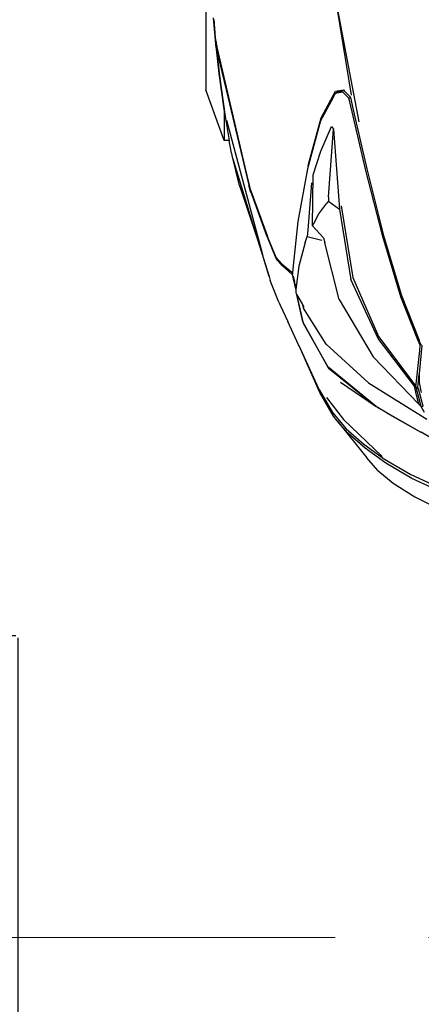
# Model space of a CAD drawing. Units: inches. Extents: x 0 to 4258, y 0 to 3769.
# Tile 5 of 30: x 3726 to 3739, y 2971 to 3003. Entities that reach past the tile are written whole.
import ezdxf

# ---------------------------------------------------------------- set-up
doc = ezdxf.new("R2010")
doc.units = ezdxf.units.IN
doc.header["$MEASUREMENT"] = 0
doc.linetypes.add('ACAD_ISO02W100', pattern=[15, 12, -3])
doc.layers.get('0').update_dxf_attribs({"color": 16})
for name, color, linetype, lineweight in [('A-ANNO-DIMS', 250, 'Continuous', 18), ('A-FLOR-OVHD', 150, 'ACAD_ISO02W100', 13), ('C-PKNG-VEHI', 8, 'Continuous', 18)]:
    doc.layers.add(name, color=color, linetype=linetype, lineweight=lineweight)
doc.layers.add('Edges', color=250, linetype='Continuous')
doc.styles.get("Standard").update_dxf_attribs({"font": 'arial.ttf'})
doc.dimstyles.get("Standard").update_dxf_attribs({"dimtxt": 7, "dimasz": 0.18, "dimexe": 0.18, "dimexo": 0.0625, "dimgap": 0.09, "dimtad": 0, "dimtih": 1, "dimtoh": 1, "dimzin": 0, "dimdsep": 46, "dimlunit": 3, "dimtxsty": 'Standard', "dimcen": 0.09, "dimadec": 0, "dimazin": 0, "dimtfac": 1, "dimtofl": 0, "dimtmove": 0, "dimatfit": 3, "dimfxl": 1, "dimtolj": 1, "dimtzin": 0, "dimarcsym": 0})

# ---------------------------------------------------------------- blocks, each defined once
blk = doc.blocks.new('Nissan Qashqai pl')
at = {"layer": 'Edges'}
for p, q in [((11.47322, 11.2592), (11.46579, 11.24614)), ((11.50736, 11.23616), (11.51652, 11.25601)), ((11.52058, 11.25724), (11.51126, 11.23721)), ((11.52949, 11.24004), (11.53843, 11.2583)), ((11.33108, 11.22699), (11.37506, 11.24429)), ((11.37475, 11.24309), (11.33228, 11.22637)), ((11.38, 11.24532), (11.37475, 11.24309)), ((11.37506, 11.24429), (11.37524, 11.24436)), ((11.37506, 11.24429), (11.37621, 11.24429)), ((11.37922, 11.24593), (11.37524, 11.24436)), ((11.3763, 11.24436), (11.37524, 11.24436)), ((11.37922, 11.24593), (11.38041, 11.24692)), ((11.37933, 11.24631), (11.37922, 11.24593)), ((11.38533, 11.24487), (11.38, 11.24532)), ((11.38041, 11.24692), (11.40818, 11.24436)), ((11.42115, 11.24117), (11.38533, 11.24487)), ((11.3915, 11.19885), (11.4381, 11.24397)), ((11.41644, 11.24436), (11.40818, 11.24436)), ((11.40898, 11.24429), (11.40818, 11.24436)), ((11.40898, 11.24429), (11.4163, 11.24429)), ((11.4152, 11.24371), (11.40898, 11.24429)), ((11.4163, 11.24429), (11.4152, 11.24371)), ((11.42154, 11.24313), (11.4152, 11.24371)), ((11.41644, 11.24436), (11.4163, 11.24429)), ((11.41686, 11.24458), (11.41644, 11.24436)), ((11.4252, 11.2462), (11.41686, 11.24458)), ((11.41698, 11.19425), (11.45295, 11.25195)), ((11.42115, 11.24117), (11.42154, 11.24313)), ((11.42296, 11.24352), (11.42154, 11.24313)), ((11.43154, 11.24397), (11.42287, 11.24164)), ((11.42296, 11.24352), (11.42287, 11.24164)), ((11.43996, 11.24823), (11.42296, 11.24352)), ((11.42659, 11.2465), (11.4252, 11.2462)), ((11.4381, 11.24397), (11.42915, 11.24177)), ((11.44027, 11.24637), (11.43154, 11.24397)), ((11.4381, 11.24397), (11.44027, 11.24637)), ((11.44027, 11.24637), (11.43996, 11.24823)), ((11.44624, 11.24948), (11.44027, 11.24637)), ((11.44114, 11.20281), (11.46562, 11.24583)), ((11.44697, 11.21272), (11.46562, 11.24583)), ((11.46562, 11.24583), (11.46579, 11.24614)), ((11.3715, 11.20434), (11.41772, 11.23895)), ((11.42033, 11.23975), (11.37334, 11.20375)), ((11.41772, 11.23895), (11.41931, 11.23998)), ((11.41915, 11.23969), (11.4194, 11.23996)), ((11.41931, 11.23998), (11.4196, 11.24017)), ((11.4194, 11.23996), (11.41931, 11.23998)), ((11.4194, 11.23996), (11.4196, 11.24017)), ((11.41958, 11.23992), (11.4194, 11.23996)), ((11.4196, 11.24017), (11.42014, 11.24052)), ((11.41984, 11.24006), (11.42014, 11.24052)), ((11.42014, 11.24052), (11.42115, 11.24117)), ((11.42915, 11.24177), (11.42033, 11.23975)), ((11.42287, 11.24164), (11.42033, 11.23975)), ((11.42178, 11.24134), (11.42115, 11.24117)), ((11.42287, 11.24164), (11.42178, 11.24134)), ((11.42216, 11.24127), (11.42178, 11.24134)), ((11.49236, 11.21027), (11.50736, 11.23616)), ((11.51126, 11.23721), (11.49628, 11.21137)), ((11.51576, 11.21859), (11.52949, 11.24004)), ((11.27199, 11.20923), (11.33108, 11.22699)), ((11.33228, 11.22637), (11.27276, 11.20843)), ((11.50327, 11.20341), (11.51576, 11.21859)), ((11.20627, 11.19262), (11.27199, 11.20923)), ((11.27276, 11.20843), (11.20665, 11.19145)), ((11.31316, 11.17892), (11.3715, 11.20434)), ((11.37334, 11.20375), (11.31527, 11.17691)), ((11.44697, 11.21272), (11.44114, 11.20281)), ((11.45306, 11.16974), (11.48975, 11.20767)), ((11.47745, 11.18983), (11.49236, 11.21027)), ((11.49628, 11.21137), (11.48154, 11.19102)), ((11.33497, 11.16556), (11.3915, 11.19885)), ((11.37896, 11.15265), (11.41698, 11.19425)), ((11.44046, 11.20182), (11.40144, 11.15414)), ((11.40216, 11.15476), (11.44046, 11.20182)), ((11.41633, 11.16662), (11.44046, 11.20182)), ((11.44081, 11.20225), (11.44046, 11.20182)), ((11.4411, 11.20277), (11.44081, 11.20225)), ((11.44114, 11.20281), (11.4411, 11.20277)), ((11.49363, 11.19502), (11.49082, 11.19282)), ((11.50327, 11.20341), (11.49363, 11.19502)), ((11.03575, 11.16129), (11.1598, 11.18473)), ((11.20665, 11.19145), (11.14012, 11.17593)), ((11.14803, 11.17913), (11.20627, 11.19262)), ((11.45433, 11.16358), (11.49082, 11.19282)), ((11.46237, 11.17248), (11.47745, 11.18983)), ((11.48154, 11.19102), (11.46617, 11.17358)), ((11.04919, 11.16347), (11.13359, 11.17719)), ((11.12929, 11.17052), (11.13526, 11.17642)), ((11.13658, 11.17502), (11.1347, 11.17313)), ((11.13526, 11.17642), (11.13585, 11.17654)), ((11.13585, 11.17654), (11.14803, 11.17913)), ((11.13585, 11.17654), (11.13658, 11.17502)), ((11.14012, 11.17593), (11.13658, 11.17502)), ((11.24278, 11.16729), (11.31316, 11.17892)), ((11.24587, 11.16563), (11.31527, 11.17691)), ((11.12846, 11.16971), (11.12929, 11.17052)), ((11.12977, 11.16183), (11.12846, 11.16971)), ((11.12929, 11.17052), (11.13057, 11.16299)), ((11.1347, 11.17313), (11.13062, 11.16899)), ((11.13062, 11.16899), (11.13192, 11.16144)), ((11.16717, 11.15976), (11.24587, 11.16563)), ((11.23823, 11.15494), (11.24587, 11.16563)), ((11.33497, 11.16556), (11.27913, 11.15147)), ((11.43143, 11.15309), (11.45306, 11.16974)), ((11.44642, 11.15882), (11.46237, 11.17248)), ((11.46617, 11.17358), (11.45433, 11.16358)), ((11.15597, 11.14759), (11.12977, 11.16183)), ((11.13192, 11.16144), (11.13057, 11.16299)), ((11.13192, 11.16144), (11.13652, 11.15905)), ((11.13652, 11.15905), (11.15893, 11.14704)), ((11.16444, 11.15792), (11.16717, 11.15976)), ((11.18896, 11.14734), (11.16444, 11.15792)), ((11.23369, 11.15498), (11.16717, 11.15976)), ((11.42433, 11.14593), (11.44642, 11.15882)), ((11.44983, 11.15977), (11.42671, 11.14629)), ((11.45433, 11.16358), (11.44983, 11.15977)), ((11.20291, 11.13489), (11.15597, 11.14759)), ((11.15893, 11.14704), (11.20616, 11.13437)), ((11.2121, 11.1399), (11.18896, 11.14734)), ((11.23369, 11.15498), (11.23823, 11.15494)), ((11.23823, 11.15494), (11.2401, 11.15337)), ((11.25046, 11.1455), (11.2401, 11.15337)), ((11.26005, 11.1405), (11.25046, 11.1455)), ((11.27429, 11.14993), (11.26224, 11.13901)), ((11.27289, 11.13379), (11.27664, 11.14845)), ((11.27429, 11.14993), (11.27913, 11.15147)), ((11.37896, 11.15265), (11.34336, 11.13032)), ((11.40144, 11.15414), (11.3571, 11.12956)), ((11.35832, 11.12998), (11.40144, 11.15414)), ((11.42671, 11.14629), (11.38067, 11.12595)), ((11.40216, 11.15476), (11.40144, 11.15414)), ((11.42283, 11.14525), (11.42433, 11.14593)), ((11.26224, 11.13901), (11.2121, 11.1399)), ((11.21991, 11.1382), (11.26663, 11.13449)), ((11.26224, 11.13901), (11.26005, 11.1405)), ((11.42283, 11.14525), (11.38067, 11.12595)), ((11.20291, 11.13489), (11.20295, 11.13488)), ((11.20295, 11.13488), (11.20616, 11.13437)), ((11.20616, 11.13437), (11.25827, 11.12461)), ((11.26663, 11.13449), (11.27289, 11.13379)), ((11.27871, 11.13184), (11.27289, 11.13379)), ((11.27871, 11.13184), (11.30218, 11.1256)), ((11.32955, 11.12347), (11.3571, 11.12956)), ((11.3571, 11.12956), (11.33021, 11.12384)), ((11.33021, 11.12384), (11.33938, 11.12898)), ((11.33938, 11.12898), (11.34202, 11.13045)), ((11.33938, 11.12898), (11.34336, 11.13032)), ((11.3571, 11.12956), (11.35832, 11.12998)), ((11.25827, 11.12461), (11.29558, 11.12077)), ((11.29558, 11.12077), (11.30849, 11.1195)), ((11.30003, 11.10916), (11.30813, 11.11883)), ((11.31027, 11.11923), (11.30178, 11.10961)), ((11.30218, 11.1256), (11.32517, 11.12286)), ((11.30805, 11.11884), (11.30863, 11.11948)), ((11.30813, 11.11883), (11.30863, 11.11948)), ((11.30849, 11.1195), (11.30863, 11.11948)), ((11.30863, 11.11948), (11.31033, 11.1193)), ((11.31033, 11.1193), (11.31027, 11.11923)), ((11.31033, 11.1193), (11.31061, 11.11927)), ((11.31061, 11.11927), (11.314, 11.12039)), ((11.31704, 11.12142), (11.31186, 11.12058)), ((11.31323, 11.11986), (11.32588, 11.12266)), ((11.32423, 11.12258), (11.314, 11.12039)), ((11.314, 11.12039), (11.31704, 11.12142)), ((11.32423, 11.12258), (11.31704, 11.12142)), ((11.31982, 11.1231), (11.32517, 11.12286)), ((11.32423, 11.12258), (11.32588, 11.12266)), ((11.32517, 11.12286), (11.32831, 11.12278)), ((11.32588, 11.12266), (11.32831, 11.12278)), ((11.32831, 11.12278), (11.32955, 11.12347)), ((11.32955, 11.12347), (11.33021, 11.12384)), ((11.37962, 11.12547), (11.35656, 11.11477)), ((11.38067, 11.12595), (11.37962, 11.12547)), ((11.29339, 11.10313), (11.30003, 11.10916)), ((11.30178, 11.10961), (11.29459, 11.10327)), ((11.33757, 11.10603), (11.34052, 11.10725)), ((11.34052, 11.10725), (11.35656, 11.11477)), ((11.29459, 11.10327), (11.27358, 11.0947)), ((11.27407, 11.09522), (11.29339, 11.10313)), ((11.31244, 11.09628), (11.31612, 11.09747)), ((11.33757, 11.10603), (11.31612, 11.09747)), ((11.15816, 11.05423), (11.29065, 11.08989)), ((11.2732, 11.09452), (11.22772, 11.07792)), ((11.23038, 11.07923), (11.27187, 11.09432)), ((11.27187, 11.09432), (11.27407, 11.09522)), ((11.27358, 11.0947), (11.2732, 11.09452)), ((11.27358, 11.0947), (11.27407, 11.09522)), ((11.27568, 11.08503), (11.31244, 11.09628)), ((11.31244, 11.09628), (11.29065, 11.08989)), ((11.30801, 11.09508), (11.30877, 11.09528)), ((11.19633, 11.06072), (11.27568, 11.08503)), ((11.22715, 11.07771), (11.2222, 11.07656)), ((11.22475, 11.06772), (11.27568, 11.08503)), ((11.22532, 11.07737), (11.23038, 11.07923)), ((11.22731, 11.07783), (11.22706, 11.07777)), ((11.22962, 11.07837), (11.22715, 11.07771)), ((11.22772, 11.07792), (11.22715, 11.07771)), ((11.22962, 11.07837), (11.22772, 11.07792)), ((11.08649, 11.04496), (11.21998, 11.07614)), ((11.22216, 11.0766), (11.08821, 11.045)), ((11.09177, 11.04531), (11.22216, 11.0766)), ((11.21998, 11.07614), (11.22216, 11.0766)), ((11.2222, 11.07656), (11.22216, 11.0766)), ((11.22238, 11.07665), (11.2222, 11.07656)), ((11.22238, 11.07665), (11.22532, 11.07737)), ((11.19065, 11.05923), (11.17828, 11.05716)), ((11.19089, 11.05929), (11.19065, 11.05923)), ((11.19089, 11.05929), (11.19297, 11.05964)), ((11.19297, 11.05964), (11.22148, 11.06662)), ((11.22148, 11.06662), (11.22475, 11.06772)), ((11.14751, 11.05208), (11.11234, 11.04716)), ((11.11474, 11.04762), (11.15472, 11.05317)), ((11.17828, 11.05208), (11.12828, 11.03408)), ((11.15248, 11.05278), (11.14751, 11.05208)), ((11.14751, 11.05208), (11.17828, 11.05208)), ((11.15472, 11.05317), (11.15248, 11.05278)), ((11.15472, 11.05317), (11.17828, 11.05716)), ((11.17828, 11.05716), (11.17828, 11.05208)), ((11.07977, 11.04339), (11.05762, 11.04159)), ((11.05899, 11.04188), (11.07681, 11.04337)), ((11.07681, 11.04337), (11.08106, 11.04371)), ((11.08696, 11.04422), (11.07977, 11.04339)), ((11.08106, 11.04371), (11.08273, 11.0441)), ((11.08114, 11.04436), (11.08208, 11.0442)), ((11.08273, 11.0441), (11.08562, 11.04476)), ((11.08273, 11.0441), (11.08365, 11.04395)), ((11.08821, 11.045), (11.08365, 11.04395)), ((11.08365, 11.04395), (11.08696, 11.04422)), ((11.08562, 11.04476), (11.08649, 11.04496)), ((11.08649, 11.04496), (11.08796, 11.04514)), ((11.08696, 11.04422), (11.08721, 11.04424)), ((11.08728, 11.04426), (11.08721, 11.04424)), ((11.08728, 11.04426), (11.08834, 11.04438)), ((11.08834, 11.04438), (11.11474, 11.04762)), ((11.11234, 11.04716), (11.08834, 11.04438)), ((10.95773, 11.03408), (11.12828, 11.03408))]:
    blk.add_line(p, q, dxfattribs=at)
blk = doc.blocks.new('car')
blk.add_blockref('Nissan Qashqai pl', (-9.74328, -11.91512))
blk = doc.blocks.new('*D66')
at = {"layer": 'A-ANNO-DIMS', "color": 0, "lineweight": -2, "transparency": 16777216}
for p, q in [((3725.517, 3125.846), (3703.936, 3125.846)), ((3704.116, 3125.666), (3704.116, 3058.01)), ((3704.116, 2982.935), (3704.116, 3050.591)), ((3725.517, 2982.755), (3703.936, 2982.755))]:
    blk.add_line(p, q, dxfattribs=at)
at = {"layer": 'A-ANNO-DIMS', "color": 0, "transparency": 16777216}
for points in [[(3704.086, 3125.666), (3704.146, 3125.666), (3704.116, 3125.846)], [(3704.086, 2982.935), (3704.146, 2982.935), (3704.116, 2982.755)]]:
    blk.add_solid(points, dxfattribs=at)
at = {"layer": 'Defpoints', "color": 0, "transparency": 16777216}
for p in [(3725.58, 3125.846), (3704.116, 2982.755), (3725.58, 2982.755)]:
    blk.add_point(p, dxfattribs=at)
at = {"layer": 'A-ANNO-DIMS', "color": 0, "transparency": 16777216, "insert": (3704.116, 3054.301), "char_height": 7, "attachment_point": 5}
blk.add_mtext('\\A1;CAR 11\'-11"', dxfattribs=at)
blk = doc.blocks.new('*D67')
at = {"layer": 'A-ANNO-DIMS', "color": 0, "lineweight": -2, "transparency": 16777216}
for p, q in [((3725.58, 2982.693), (3725.58, 2961.112)), ((3795.713, 2982.693), (3795.713, 2961.112)), ((3725.76, 2961.292), (3748.533, 2961.292)), ((3795.533, 2961.292), (3772.76, 2961.292))]:
    blk.add_line(p, q, dxfattribs=at)
at = {"layer": 'A-ANNO-DIMS', "color": 0, "transparency": 16777216}
for points in [[(3725.76, 2961.322), (3725.76, 2961.262), (3725.58, 2961.292)], [(3795.533, 2961.322), (3795.533, 2961.262), (3795.713, 2961.292)]]:
    blk.add_solid(points, dxfattribs=at)
at = {"layer": 'Defpoints', "color": 0, "transparency": 16777216}
for p in [(3725.58, 2982.755), (3795.713, 2982.755), (3795.713, 2961.292)]:
    blk.add_point(p, dxfattribs=at)
at = {"layer": 'A-ANNO-DIMS', "color": 0, "transparency": 16777216, "insert": (3760.646, 2961.292), "char_height": 7, "attachment_point": 5}
blk.add_mtext('\\A1;5\'-10"', dxfattribs=at)

msp = doc.modelspace()

# ---------------------------------------------------------------- linework, layer by layer
at = {"layer": 'A-FLOR-OVHD'}
msp.add_line((3678.804, 2973.052), (3832.744, 2973.052), dxfattribs=at)

# ---------------------------------------------------------------- block references
at = {"layer": 'C-PKNG-VEHI', "xscale": 32.66500240257601, "yscale": 32.66500240257601, "zscale": 32.66500240257601, "rotation": 270}
msp.add_blockref('car', (3760.419, 3045.57), dxfattribs=at)

# ---------------------------------------------------------------- dimensions: what is measured, and where the dimension line sits
at = {"layer": 'A-ANNO-DIMS'}
dim = msp.add_linear_dim(base=(3704.116, 2982.755), p1=(3725.58, 3125.846), p2=(3725.58, 2982.755), angle=270, text='CAR <>', dimstyle='Standard', override={"dimdec": 1, "dimlfac": 1, "dimrnd": 0, "dimzin": 1, "dimdsep": 46, "dimlunit": 4, "dimfrac": 2}, dxfattribs=at)
dim.commit()
dim.dimension.update_dxf_attribs({"geometry": '*D66', "text_midpoint": (3704.116, 3054.301)})
dim = msp.add_linear_dim(base=(3795.713, 2961.292), p1=(3725.58, 2982.755), p2=(3795.713, 2982.755), dimstyle='Standard', override={"dimdec": 1, "dimlfac": 1, "dimrnd": 0, "dimzin": 1, "dimdsep": 46, "dimlunit": 4, "dimfrac": 2}, dxfattribs=at)
dim.commit()
dim.dimension.update_dxf_attribs({"geometry": '*D67', "text_midpoint": (3760.646, 2961.292)})

doc.saveas('drawing.dxf')
